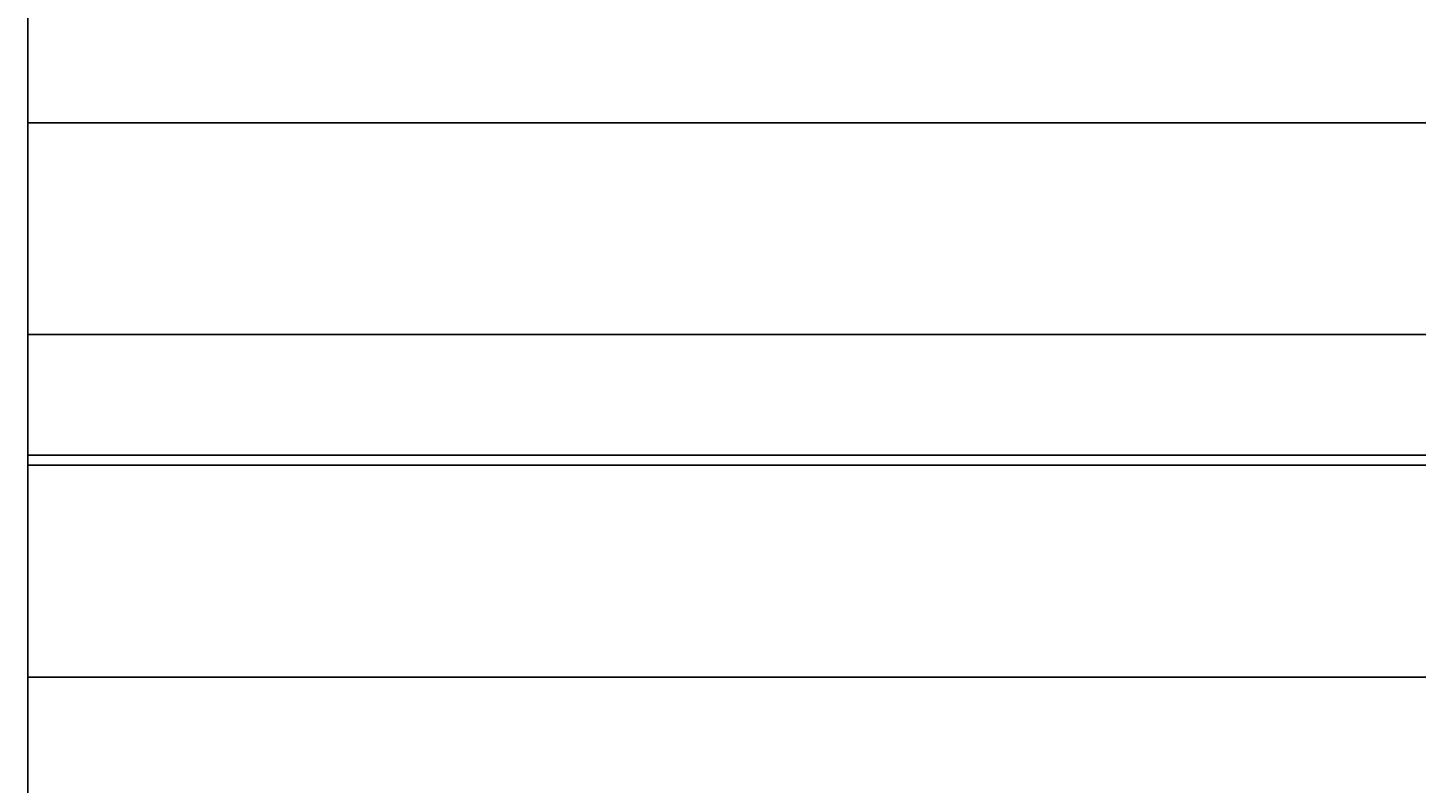
# Model space of a CAD drawing. Units: inches. Extents: x 35362 to 73946, y 43607 to 67532.
# Tile 14 of 134: x 35362 to 46225, y 50863 to 56772. Entities that reach past the tile are written whole.
import ezdxf

# ---------------------------------------------------------------- set-up
doc = ezdxf.new("R2010")
doc.units = ezdxf.units.IN
doc.header["$MEASUREMENT"] = 0
doc.layers.add('A-ANNO-DIMS', color=2, linetype='Continuous', lineweight=18)
doc.styles.get("Standard").update_dxf_attribs({"font": 'arial.ttf'})
doc.dimstyles.get("Standard").update_dxf_attribs({"dimtxt": 0.18, "dimasz": 0.18, "dimexe": 0.18, "dimexo": 0.0625, "dimgap": 0.09, "dimtad": 0, "dimtih": 1, "dimtoh": 1, "dimdec": 4, "dimzin": 0, "dimdsep": 46, "dimtxsty": 'Standard', "dimcen": 0.09, "dimadec": 0, "dimazin": 0, "dimtfac": 1, "dimtdec": 4, "dimtofl": 0, "dimtmove": 0, "dimatfit": 3, "dimfxl": 1, "dimtolj": 1, "dimtzin": 0, "dimarcsym": 0})

# ---------------------------------------------------------------- blocks, each defined once
blk = doc.blocks.new('*D12')
at = {"layer": 'A-ANNO-DIMS', "color": 0, "lineweight": -2, "transparency": 16777216}
for p, q in [((47978.60234600001, 59023.27631300003), (35361.76908500003, 59023.27631300003)), ((35361.94908500003, 59023.09631300003), (35361.94908500003, 57526.23819563782)), ((35361.94908500003, 56029.01627200003), (35361.94908500003, 57525.87438936224)), ((47978.60234600001, 56028.83627200003), (35361.76908500003, 56028.83627200003))]:
    blk.add_line(p, q, dxfattribs=at)
at = {"layer": 'A-ANNO-DIMS', "color": 0, "transparency": 16777216}
for points in [[(35361.91908500003, 59023.09631300003), (35361.97908500003, 59023.09631300003), (35361.94908500003, 59023.27631300003)], [(35361.91908500003, 56029.01627200003), (35361.97908500003, 56029.01627200003), (35361.94908500003, 56028.83627200003)]]:
    blk.add_solid(points, dxfattribs=at)
at = {"layer": 'Defpoints', "color": 0, "transparency": 16777216}
for p in [(47978.66484600001, 59023.27631300003), (35361.94908500003, 56028.83627200003), (47978.66484600001, 56028.83627200003)]:
    blk.add_point(p, dxfattribs=at)
at = {"layer": 'A-ANNO-DIMS', "color": 0, "transparency": 16777216, "insert": (35361.94908500004, 57526.05629250001), "char_height": 0.18, "attachment_point": 5}
blk.add_mtext('\\A1;2994.4', dxfattribs=at)
blk = doc.blocks.new('*D14')
at = {"layer": 'A-ANNO-DIMS', "color": 0, "lineweight": -2, "transparency": 16777216}
for p, q in [((48373.42909800002, 53429.01856500002), (35361.76908500003, 53429.01856500002)), ((35361.94908500003, 53428.83856500002), (35361.94908500003, 52561.73476102936)), ((35361.94908500003, 51694.26702800003), (35361.94908500003, 52561.3708319707)), ((48373.42909800002, 51694.08702800003), (35361.76908500003, 51694.08702800003))]:
    blk.add_line(p, q, dxfattribs=at)
at = {"layer": 'A-ANNO-DIMS', "color": 0, "transparency": 16777216}
for points in [[(35361.91908500003, 53428.83856500002), (35361.97908500003, 53428.83856500002), (35361.94908500003, 53429.01856500002)], [(35361.91908500003, 51694.26702800003), (35361.97908500003, 51694.26702800003), (35361.94908500003, 51694.08702800003)]]:
    blk.add_solid(points, dxfattribs=at)
at = {"layer": 'Defpoints', "color": 0, "transparency": 16777216}
for p in [(48373.49159800001, 53429.01856500002), (35361.94908500003, 51694.08702800003), (48373.49159800001, 51694.08702800003)]:
    blk.add_point(p, dxfattribs=at)
at = {"layer": 'A-ANNO-DIMS', "color": 0, "transparency": 16777216, "insert": (35361.94908500004, 52561.5527965), "char_height": 0.18, "attachment_point": 5}
blk.add_mtext('\\A1;1735', dxfattribs=at)
blk = doc.blocks.new('*D26')
at = {"layer": 'A-ANNO-DIMS', "color": 0, "lineweight": -2, "transparency": 16777216}
for p, q in [((47978.60234600001, 56028.83627200003), (35361.76908500003, 56028.83627200003)), ((35361.94908500003, 56028.65627200003), (35361.94908500003, 54729.10932163782)), ((35361.94908500003, 53429.19856500002), (35361.94908500003, 54728.74551536224)), ((48373.42909800002, 53429.01856500002), (35361.76908500003, 53429.01856500002))]:
    blk.add_line(p, q, dxfattribs=at)
at = {"layer": 'A-ANNO-DIMS', "color": 0, "transparency": 16777216}
for points in [[(35361.91908500003, 56028.65627200003), (35361.97908500003, 56028.65627200003), (35361.94908500003, 56028.83627200003)], [(35361.91908500003, 53429.19856500002), (35361.97908500003, 53429.19856500002), (35361.94908500003, 53429.01856500002)]]:
    blk.add_solid(points, dxfattribs=at)
at = {"layer": 'Defpoints', "color": 0, "transparency": 16777216}
for p in [(35361.94908500003, 56028.83627200003), (47978.66484600001, 56028.83627200003), (48373.49159800001, 53429.01856500002)]:
    blk.add_point(p, dxfattribs=at)
at = {"layer": 'A-ANNO-DIMS', "color": 0, "transparency": 16777216, "insert": (35361.94908500004, 54728.92741850001), "char_height": 0.18, "attachment_point": 5}
blk.add_mtext('\\A1;2599.8', dxfattribs=at)
blk = doc.blocks.new('*D36')
at = {"layer": 'A-ANNO-DIMS', "color": 0, "lineweight": -2, "transparency": 16777216}
for p, q in [((68320.80826200004, 60122.34633200002), (35361.76908500003, 60122.34633200002)), ((35361.94908500003, 60122.16633200002), (35361.94908500003, 57247.82893113781)), ((35361.94908500003, 54373.12772400002), (35361.94908500003, 57247.46512486223)), ((68320.80826200004, 54372.94772400003), (35361.76908500003, 54372.94772400002))]:
    blk.add_line(p, q, dxfattribs=at)
at = {"layer": 'A-ANNO-DIMS', "color": 0, "transparency": 16777216}
for points in [[(35361.91908500003, 60122.16633200002), (35361.97908500003, 60122.16633200002), (35361.94908500003, 60122.34633200002)], [(35361.91908500003, 54373.12772400002), (35361.97908500003, 54373.12772400002), (35361.94908500003, 54372.94772400002)]]:
    blk.add_solid(points, dxfattribs=at)
at = {"layer": 'Defpoints', "color": 0, "transparency": 16777216}
for p in [(68320.87076200004, 60122.34633200002), (35361.94908500003, 54372.94772400002), (68320.87076200004, 54372.94772400003)]:
    blk.add_point(p, dxfattribs=at)
at = {"layer": 'A-ANNO-DIMS', "color": 0, "transparency": 16777216, "insert": (35361.94908500004, 57247.64702799999), "char_height": 0.18, "attachment_point": 5}
blk.add_mtext('\\A1;5749.4', dxfattribs=at)
blk = doc.blocks.new('*D40')
at = {"layer": 'A-ANNO-DIMS', "color": 0, "lineweight": -2, "transparency": 16777216}
for p, q in [((56873.53943900003, 53351.52866200003), (35361.76908500003, 53351.52866200002)), ((35361.94908500003, 53351.34866200002), (35361.94908500003, 51333.28097302935)), ((35361.94908500003, 49314.84935500002), (35361.94908500003, 51332.91704397068)), ((51806.45408000003, 49314.66935500003), (35361.76908500003, 49314.66935500002))]:
    blk.add_line(p, q, dxfattribs=at)
at = {"layer": 'A-ANNO-DIMS', "color": 0, "transparency": 16777216}
for points in [[(35361.91908500003, 53351.34866200002), (35361.97908500003, 53351.34866200002), (35361.94908500003, 53351.52866200002)], [(35361.91908500003, 49314.84935500002), (35361.97908500003, 49314.84935500002), (35361.94908500003, 49314.66935500002)]]:
    blk.add_solid(points, dxfattribs=at)
at = {"layer": 'Defpoints', "color": 0, "transparency": 16777216}
for p in [(35361.94908500003, 53351.52866200002), (56873.60193900003, 53351.52866200003), (51806.51658000003, 49314.66935500003)]:
    blk.add_point(p, dxfattribs=at)
at = {"layer": 'A-ANNO-DIMS', "color": 0, "transparency": 16777216, "insert": (35361.94908500004, 51333.09900849999), "char_height": 0.18, "attachment_point": 5}
blk.add_mtext('\\A1;4036.9', dxfattribs=at)
blk = doc.blocks.new('*D67')
at = {"layer": 'A-ANNO-DIMS', "color": 0, "lineweight": -2, "transparency": 16777216}
for p, q in [((56873.53943900003, 53351.52866200003), (35361.76908500003, 53351.52866200002)), ((35361.94908500003, 53351.34866200002), (35361.94908500003, 49400.89345963781)), ((35361.94908500004, 45450.07445100001), (35361.94908500003, 49400.52965336223)), ((53793.57528900003, 45449.89445100001), (35361.76908500004, 45449.894451))]:
    blk.add_line(p, q, dxfattribs=at)
at = {"layer": 'A-ANNO-DIMS', "color": 0, "transparency": 16777216}
for points in [[(35361.91908500003, 53351.34866200002), (35361.97908500003, 53351.34866200002), (35361.94908500003, 53351.52866200002)], [(35361.91908500004, 45450.07445100001), (35361.97908500004, 45450.07445100001), (35361.94908500004, 45449.894451)]]:
    blk.add_solid(points, dxfattribs=at)
at = {"layer": 'Defpoints', "color": 0, "transparency": 16777216}
for p in [(35361.94908500003, 53351.52866200002), (56873.60193900003, 53351.52866200003), (53793.63778900002, 45449.89445100001)]:
    blk.add_point(p, dxfattribs=at)
at = {"layer": 'A-ANNO-DIMS', "color": 0, "transparency": 16777216, "insert": (35361.94908500004, 49400.7115565), "char_height": 0.18, "attachment_point": 5}
blk.add_mtext('\\A1;7901.6', dxfattribs=at)

msp = doc.modelspace()

# ---------------------------------------------------------------- dimensions: what is measured, and where the dimension line sits
at = {"layer": 'A-ANNO-DIMS'}
for base, p1, p2, override, picture, middle in [((35361.94908500003, 54372.94772400002), (68320.870762, 60122.346332), (68320.870762, 54372.947724), {"dimdec": 1, "dimlfac": 1, "dimrnd": 0, "dimzin": 0, "dimdsep": 46, "dimlunit": 2}, '*D36', (35361.94908500004, 57247.64702799999)), ((35361.94908500003, 56028.83627200003), (47978.664846, 59023.276313), (47978.664846, 56028.836272), {"dimdec": 1, "dimlfac": 1, "dimrnd": 0, "dimzin": 0, "dimdsep": 46, "dimlunit": 2}, '*D12', (35361.94908500004, 57526.05629250001)), ((35361.94908500003, 56028.83627200003), (48373.491598, 53429.018565), (47978.664846, 56028.836272), {"dimdec": 1, "dimlfac": 1, "dimrnd": 0, "dimzin": 0, "dimdsep": 46, "dimlunit": 2}, '*D26', (35361.94908500004, 54728.92741850001)), ((35361.94908500003, 53351.52866200002), (51806.51658, 49314.669355), (56873.601939, 53351.52866199999), {"dimdec": 1, "dimlfac": 1, "dimrnd": 0, "dimzin": 0, "dimdsep": 46, "dimlunit": 2}, '*D40', (35361.94908500004, 51333.09900849999)), ((35361.94908500003, 53351.52866200002), (53793.637789, 45449.894451), (56873.601939, 53351.52866199999), {"dimdec": 1, "dimlfac": 1, "dimrnd": 0, "dimzin": 0, "dimdsep": 46, "dimlunit": 2}, '*D67', (35361.94908500004, 49400.7115565)), ((35361.94908500003, 51694.08702800003), (48373.491598, 53429.018565), (48373.491598, 51694.087028), {"dimdec": 0, "dimlfac": 1, "dimrnd": 0, "dimzin": 0, "dimdsep": 46, "dimlunit": 2}, '*D14', (35361.94908500004, 52561.5527965))]:
    dim = msp.add_linear_dim(base=base, p1=p1, p2=p2, angle=90, dimstyle='Standard', override=override, dxfattribs=at)
    dim.commit()
    dim.dimension.update_dxf_attribs({"geometry": picture, "text_midpoint": middle})

doc.saveas('drawing.dxf')
